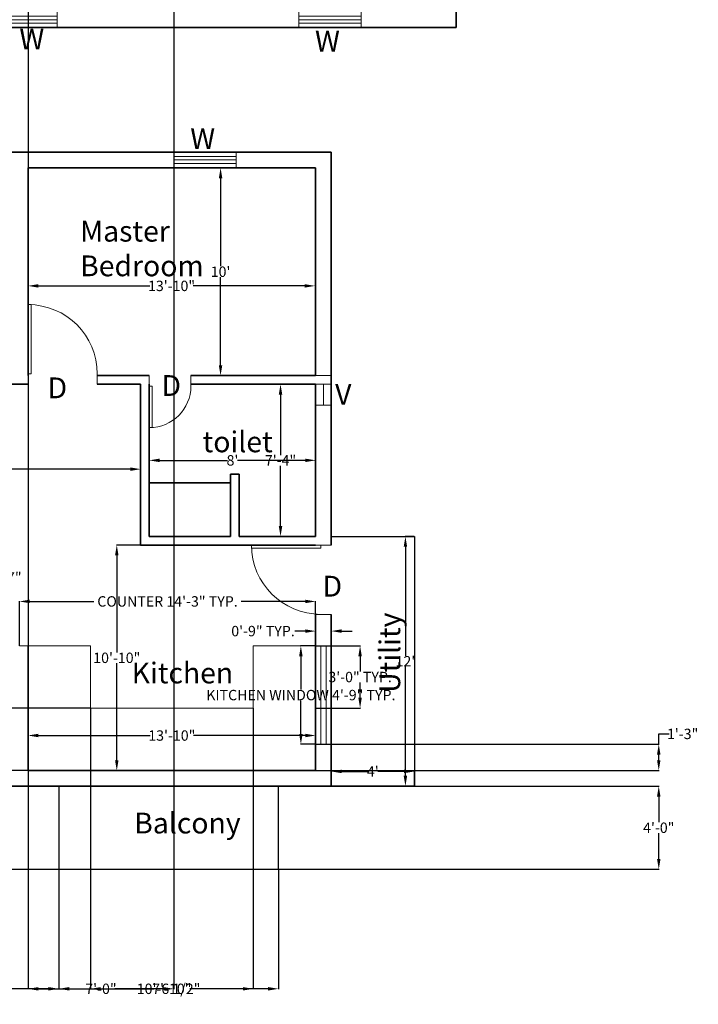
# Model space of a CAD drawing. Units: inches. Extents: x 1936 to 2761, y 1431 to 2889.
# Tile 2 of 6: x 2369 to 2761, y 1431 to 1999. Entities that reach past the tile are written whole.
import ezdxf

# ---------------------------------------------------------------- set-up
doc = ezdxf.new("R2010")
doc.units = ezdxf.units.IN
doc.header["$MEASUREMENT"] = 0
for name, color, linetype, lineweight in [('A-ANNO-DIMS', 172, 'Continuous', 13), ('A-ANNO-TEXT', 50, 'Continuous', 18), ('A-AREA-IDEN', 50, 'Continuous', 18), ('A-FLOR-EDGE', 4, 'Continuous', 25), ('A-FLOR-FIXT', 8, 'Continuous', 18), ('A-GLAZ', 3, 'Continuous', 18), ('A-WALL', 4, 'Continuous', 35), ('doors', 10, 'Continuous', 18)]:
    doc.layers.add(name, color=color, linetype=linetype, lineweight=lineweight)
doc.styles.get("Standard").update_dxf_attribs({"font": 'arial.ttf'})
doc.dimstyles.get("Standard").update_dxf_attribs({"dimtxt": 6, "dimasz": 6, "dimexe": 0.18, "dimexo": 0.0625, "dimgap": 0.09, "dimtad": 0, "dimtih": 1, "dimtoh": 1, "dimdec": 0, "dimzin": 0, "dimdsep": 46, "dimlunit": 3, "dimtxsty": 'Standard', "dimcen": 0.09, "dimadec": 0, "dimazin": 0, "dimtfac": 1, "dimtdec": 0, "dimtofl": 0, "dimtmove": 0, "dimatfit": 3, "dimfxl": 1, "dimtolj": 1, "dimtzin": 0, "dimarcsym": 0})

# ---------------------------------------------------------------- blocks, each defined once
blk = doc.blocks.new('*U2')
for p, q in [((0, 0), (0, 6)), ((40, 0), (40, 6))]:
    blk.add_line(p, q)
blk.add_lwpolyline([(0, 0), (0, -40), (1.75, -40), (1.75, 0)], close=True)
blk.add_arc((0, 0), 40, 270, 360)
blk = doc.blocks.new('*U3')
for p, q in [((0, 0), (0, -6)), ((24, 0), (24, -6))]:
    blk.add_line(p, q)
blk.add_lwpolyline([(0, 0), (0, 24), (1.75, 24), (1.75, 0)], close=True)
blk.add_arc((0, 0), 24, 0, 90)
blk = doc.blocks.new('*U5')
for p, q in [((0, 0), (0, -6)), ((40, 0), (40, -6))]:
    blk.add_line(p, q)
blk.add_lwpolyline([(0, 0), (0, 40), (1.75, 40), (1.75, 0)], close=True)
blk.add_arc((0, 0), 40, 0, 90)
blk = doc.blocks.new('*D59')
at = {"layer": 'A-ANNO-DIMS', "color": 0, "lineweight": -2, "transparency": 16777216}
for p, q in [((2249.01, 1739.61), (2249.01, 1739.73)), ((2255.01, 1739.55), (2331.56, 1739.55)), ((2433.01, 1739.55), (2356.45, 1739.55)), ((2439.01, 1739.61), (2439.01, 1739.73))]:
    blk.add_line(p, q, dxfattribs=at)
at = {"layer": 'A-ANNO-DIMS', "color": 0, "transparency": 16777216}
for points in [[(2255.01, 1740.55), (2255.01, 1738.55), (2249.01, 1739.55)], [(2433.01, 1740.55), (2433.01, 1738.55), (2439.01, 1739.55)]]:
    blk.add_solid(points, dxfattribs=at)
at = {"layer": 'Defpoints', "color": 0, "transparency": 16777216}
for p in [(2249.01, 1739.55), (2439.01, 1739.55), (2439.01, 1739.55)]:
    blk.add_point(p, dxfattribs=at)
at = {"layer": 'A-ANNO-DIMS', "color": 0, "transparency": 16777216, "insert": (2344.01, 1739.55), "char_height": 6, "attachment_point": 5}
blk.add_mtext('\\A1;15\'-10"', dxfattribs=at)
blk = doc.blocks.new('*D60')
at = {"layer": 'A-ANNO-DIMS', "color": 0, "lineweight": -2, "transparency": 16777216}
for p, q in [((2347.57, 1788.55), (2359.19, 1788.55)), ((2359.01, 1782.55), (2359.01, 1680.2)), ((2359.01, 1571.55), (2359.01, 1673.9)), ((2347.57, 1565.55), (2359.19, 1565.55))]:
    blk.add_line(p, q, dxfattribs=at)
at = {"layer": 'A-ANNO-DIMS', "color": 0, "transparency": 16777216}
for points in [[(2358.01, 1782.55), (2360.01, 1782.55), (2359.01, 1788.55)], [(2358.01, 1571.55), (2360.01, 1571.55), (2359.01, 1565.55)]]:
    blk.add_solid(points, dxfattribs=at)
at = {"layer": 'Defpoints', "color": 0, "transparency": 16777216}
for p in [(2347.51, 1788.55), (2359.01, 1788.55), (2347.51, 1565.55)]:
    blk.add_point(p, dxfattribs=at)
at = {"layer": 'A-ANNO-DIMS', "color": 0, "transparency": 16777216, "insert": (2359.01, 1677.05), "char_height": 6, "attachment_point": 5}
blk.add_mtext('\\A1;18\'-7"', dxfattribs=at)
blk = doc.blocks.new('*D61')
at = {"layer": 'A-ANNO-DIMS', "color": 0, "lineweight": -2, "transparency": 16777216}
for p, q in [((2374.01, 1585.84), (2374.01, 1585.96)), ((2380.01, 1585.78), (2444.56, 1585.78)), ((2534.01, 1585.78), (2469.45, 1585.78)), ((2540.01, 1585.84), (2540.01, 1585.96))]:
    blk.add_line(p, q, dxfattribs=at)
at = {"layer": 'A-ANNO-DIMS', "color": 0, "transparency": 16777216}
for points in [[(2380.01, 1586.78), (2380.01, 1584.78), (2374.01, 1585.78)], [(2534.01, 1586.78), (2534.01, 1584.78), (2540.01, 1585.78)]]:
    blk.add_solid(points, dxfattribs=at)
at = {"layer": 'Defpoints', "color": 0, "transparency": 16777216}
for p in [(2374.01, 1585.78), (2540.01, 1585.78), (2540.01, 1585.78)]:
    blk.add_point(p, dxfattribs=at)
at = {"layer": 'A-ANNO-DIMS', "color": 0, "transparency": 16777216, "insert": (2457.01, 1585.78), "char_height": 6, "attachment_point": 5}
blk.add_mtext('\\A1;13\'-10"', dxfattribs=at)
blk = doc.blocks.new('*D62')
at = {"layer": 'A-ANNO-DIMS', "color": 0, "lineweight": -2, "transparency": 16777216}
for p, q in [((2489.44, 1695.74), (2425.06, 1695.74)), ((2425.24, 1689.74), (2425.24, 1633.8)), ((2425.24, 1571.55), (2425.24, 1627.49)), ((2485.38, 1565.55), (2425.06, 1565.55))]:
    blk.add_line(p, q, dxfattribs=at)
at = {"layer": 'A-ANNO-DIMS', "color": 0, "transparency": 16777216}
for points in [[(2424.24, 1689.74), (2426.24, 1689.74), (2425.24, 1695.74)], [(2424.24, 1571.55), (2426.24, 1571.55), (2425.24, 1565.55)]]:
    blk.add_solid(points, dxfattribs=at)
at = {"layer": 'Defpoints', "color": 0, "transparency": 16777216}
for p in [(2425.24, 1695.74), (2489.51, 1695.74), (2485.44, 1565.55)]:
    blk.add_point(p, dxfattribs=at)
at = {"layer": 'A-ANNO-DIMS', "color": 0, "transparency": 16777216, "insert": (2425.24, 1630.64), "char_height": 6, "attachment_point": 5}
blk.add_mtext('\\A1;10\'-10"', dxfattribs=at)
blk = doc.blocks.new('*D63')
at = {"layer": 'A-ANNO-DIMS', "color": 0, "lineweight": -2, "transparency": 16777216}
for p, q in [((2444.01, 1744.58), (2444.01, 1744.46)), ((2450.01, 1744.64), (2489.15, 1744.64)), ((2534.01, 1744.64), (2494.86, 1744.64)), ((2540.01, 1744.71), (2540.01, 1744.82))]:
    blk.add_line(p, q, dxfattribs=at)
at = {"layer": 'A-ANNO-DIMS', "color": 0, "transparency": 16777216}
for points in [[(2450.01, 1745.64), (2450.01, 1743.64), (2444.01, 1744.64)], [(2534.01, 1745.64), (2534.01, 1743.64), (2540.01, 1744.64)]]:
    blk.add_solid(points, dxfattribs=at)
at = {"layer": 'Defpoints', "color": 0, "transparency": 16777216}
for p in [(2444.01, 1744.64), (2540.01, 1744.64), (2540.01, 1744.64)]:
    blk.add_point(p, dxfattribs=at)
at = {"layer": 'A-ANNO-DIMS', "color": 0, "transparency": 16777216, "insert": (2492.01, 1744.64), "char_height": 6, "attachment_point": 5}
blk.add_mtext("\\A1;8'", dxfattribs=at)
blk = doc.blocks.new('*D64')
at = {"layer": 'A-ANNO-DIMS', "color": 0, "lineweight": -2, "transparency": 16777216}
for p, q in [((2518.02, 1788.55), (2519.92, 1788.55)), ((2519.74, 1782.55), (2519.74, 1747.73)), ((2519.74, 1706.74), (2519.74, 1741.55)), ((2518.02, 1700.74), (2519.92, 1700.74))]:
    blk.add_line(p, q, dxfattribs=at)
at = {"layer": 'A-ANNO-DIMS', "color": 0, "transparency": 16777216}
for points in [[(2518.74, 1782.55), (2520.74, 1782.55), (2519.74, 1788.55)], [(2518.74, 1706.74), (2520.74, 1706.74), (2519.74, 1700.74)]]:
    blk.add_solid(points, dxfattribs=at)
at = {"layer": 'Defpoints', "color": 0, "transparency": 16777216}
for p in [(2517.96, 1788.55), (2519.74, 1788.55), (2517.96, 1700.74)]:
    blk.add_point(p, dxfattribs=at)
at = {"layer": 'A-ANNO-DIMS', "color": 0, "transparency": 16777216, "insert": (2519.74, 1744.64), "char_height": 6, "attachment_point": 5}
blk.add_mtext('\\A1;7\'-4"', dxfattribs=at)
blk = doc.blocks.new('*D73')
at = {"layer": 'A-ANNO-DIMS', "color": 0, "lineweight": -2, "transparency": 16777216}
for p, q in [((2374.01, 1858), (2374.01, 1845.18)), ((2539.69, 1858), (2539.69, 1845.18)), ((2380.01, 1845.36), (2444.41, 1845.36)), ((2533.69, 1845.36), (2469.29, 1845.36))]:
    blk.add_line(p, q, dxfattribs=at)
at = {"layer": 'A-ANNO-DIMS', "color": 0, "transparency": 16777216}
for points in [[(2380.01, 1846.36), (2380.01, 1844.36), (2374.01, 1845.36)], [(2533.69, 1846.36), (2533.69, 1844.36), (2539.69, 1845.36)]]:
    blk.add_solid(points, dxfattribs=at)
at = {"layer": 'Defpoints', "color": 0, "transparency": 16777216}
for p in [(2374.01, 1858.06), (2539.69, 1858.06), (2374.01, 1845.36)]:
    blk.add_point(p, dxfattribs=at)
at = {"layer": 'A-ANNO-DIMS', "color": 0, "transparency": 16777216, "insert": (2456.85, 1845.36), "char_height": 6, "attachment_point": 5}
blk.add_mtext('\\A1;13\'-10"', dxfattribs=at)
blk = doc.blocks.new('*D74')
at = {"layer": 'A-ANNO-DIMS', "color": 0, "lineweight": -2, "transparency": 16777216}
for p, q in [((2480.34, 1913.55), (2485.32, 1913.55)), ((2485.14, 1907.55), (2485.14, 1856.7)), ((2485.14, 1799.55), (2485.14, 1850.4)), ((2480.34, 1793.55), (2485.32, 1793.55))]:
    blk.add_line(p, q, dxfattribs=at)
at = {"layer": 'A-ANNO-DIMS', "color": 0, "transparency": 16777216}
for points in [[(2484.14, 1907.55), (2486.14, 1907.55), (2485.14, 1913.55)], [(2484.14, 1799.55), (2486.14, 1799.55), (2485.14, 1793.55)]]:
    blk.add_solid(points, dxfattribs=at)
at = {"layer": 'Defpoints', "color": 0, "transparency": 16777216}
for p in [(2480.28, 1913.55), (2480.28, 1793.55), (2485.14, 1793.55)]:
    blk.add_point(p, dxfattribs=at)
at = {"layer": 'A-ANNO-DIMS', "color": 0, "transparency": 16777216, "insert": (2485.14, 1853.55), "char_height": 6, "attachment_point": 5}
blk.add_mtext("\\A1;10'", dxfattribs=at)
blk = doc.blocks.new('*D56')
at = {"layer": 'A-ANNO-DIMS', "color": 0, "lineweight": -2, "transparency": 16777216}
for p, q in [((2549.01, 1556.61), (2549.01, 1565.24)), ((2555.01, 1565.06), (2570.03, 1565.06)), ((2591.01, 1565.06), (2575.98, 1565.06)), ((2597.01, 1556.61), (2597.01, 1565.24))]:
    blk.add_line(p, q, dxfattribs=at)
at = {"layer": 'A-ANNO-DIMS', "color": 0, "transparency": 16777216}
for points in [[(2555.01, 1566.06), (2555.01, 1564.06), (2549.01, 1565.06)], [(2591.01, 1566.06), (2591.01, 1564.06), (2597.01, 1565.06)]]:
    blk.add_solid(points, dxfattribs=at)
at = {"layer": 'Defpoints', "color": 0, "transparency": 16777216}
for p in [(2597.01, 1565.06), (2549.01, 1556.55), (2597.01, 1556.55)]:
    blk.add_point(p, dxfattribs=at)
at = {"layer": 'A-ANNO-DIMS', "color": 0, "transparency": 16777216, "insert": (2573.01, 1565.06), "char_height": 6, "attachment_point": 5}
blk.add_mtext("\\A1;4'", dxfattribs=at)
blk = doc.blocks.new('*D75')
at = {"layer": 'A-ANNO-DIMS', "color": 0, "lineweight": -2, "transparency": 16777216}
for p, q in [((2596.94, 1700.74), (2591.63, 1700.74)), ((2591.81, 1694.74), (2591.81, 1631.75)), ((2591.81, 1562.55), (2591.81, 1625.54)), ((2596.94, 1556.55), (2591.63, 1556.55))]:
    blk.add_line(p, q, dxfattribs=at)
at = {"layer": 'A-ANNO-DIMS', "color": 0, "transparency": 16777216}
for points in [[(2590.81, 1694.74), (2592.81, 1694.74), (2591.81, 1700.74)], [(2590.81, 1562.55), (2592.81, 1562.55), (2591.81, 1556.55)]]:
    blk.add_solid(points, dxfattribs=at)
at = {"layer": 'Defpoints', "color": 0, "transparency": 16777216}
for p in [(2591.81, 1700.74), (2597.01, 1700.74), (2597.01, 1556.55)]:
    blk.add_point(p, dxfattribs=at)
at = {"layer": 'A-ANNO-DIMS', "color": 0, "transparency": 16777216, "insert": (2591.81, 1628.64), "char_height": 6, "attachment_point": 5}
blk.add_mtext("\\A1;12'", dxfattribs=at)
blk = doc.blocks.new('WIN-36')
for p, q in [((0, 9), (0, 0)), ((36, 6.5), (0, 6.5)), ((36, 9), (36, 0)), ((36, 4.5), (0, 4.5)), ((36, 2.5), (0, 2.5))]:
    blk.add_line(p, q)
blk = doc.blocks.new('VENT-12')
for p, q in [((0, 0), (0, 9)), ((12, 0), (12, 9)), ((0, 4.5), (12, 4.5))]:
    blk.add_line(p, q)
blk = doc.blocks.new('WIN-KITCHEN')
for p, q in [((0, 56.83), (9, 56.83)), ((3, 56.83), (3, 0)), ((6, 56.83), (6, 0)), ((0, 0), (9, 0))]:
    blk.add_line(p, q)
blk = doc.blocks.new('COUNTER-KITCHEN-U')
for p, q in [((41, 36), (41, 0)), ((41, 36), (135, 36)), ((135, 36), (135, 0)), ((0, 0), (41, 0)), ((135, 0), (171, 0))]:
    blk.add_line(p, q)
blk = doc.blocks.new('BATH-PARTITION')
for p, q in [((0, 35.9), (46.9, 35.9)), ((0, 5), (0, 35.9)), ((46.9, 35.9), (46.9, 0)), ((51.9, 35.9), (51.9, 0)), ((46.9, 5), (0, 5)), ((51.9, 0), (46.9, 0))]:
    blk.add_line(p, q)
blk = doc.blocks.new('*D91')
at = {"layer": 'A-ANNO-DIMS', "color": 0, "lineweight": -2, "transparency": 16777216}
for p, q in [((2539.94, 1637.55), (2531.3, 1637.55)), ((2531.48, 1631.55), (2531.48, 1612.33)), ((2531.48, 1586.72), (2531.48, 1605.94)), ((2539.94, 1580.72), (2531.3, 1580.72))]:
    blk.add_line(p, q, dxfattribs=at)
at = {"layer": 'A-ANNO-DIMS', "color": 0, "transparency": 16777216}
for points in [[(2530.48, 1631.55), (2532.48, 1631.55), (2531.48, 1637.55)], [(2530.48, 1586.72), (2532.48, 1586.72), (2531.48, 1580.72)]]:
    blk.add_solid(points, dxfattribs=at)
at = {"layer": 'Defpoints', "color": 0, "transparency": 16777216}
for p in [(2540.01, 1637.55), (2531.48, 1580.72), (2540.01, 1580.72)]:
    blk.add_point(p, dxfattribs=at)
at = {"layer": 'A-ANNO-DIMS', "color": 0, "transparency": 16777216, "insert": (2531.48, 1609.13), "char_height": 6, "attachment_point": 5}
blk.add_mtext('\\A1;KITCHEN WINDOW 4\'-9" TYP.', dxfattribs=at)
blk = doc.blocks.new('*D92')
at = {"layer": 'A-ANNO-DIMS', "color": 0, "lineweight": -2, "transparency": 16777216}
for p, q in [((2534.01, 1646.07), (2528.01, 1646.07)), ((2540.01, 1637.61), (2540.01, 1646.25)), ((2549.01, 1637.61), (2549.01, 1646.25)), ((2555.01, 1646.07), (2561.01, 1646.07))]:
    blk.add_line(p, q, dxfattribs=at)
at = {"layer": 'A-ANNO-DIMS', "color": 0, "transparency": 16777216}
for points in [[(2534.01, 1647.07), (2534.01, 1645.07), (2540.01, 1646.07)], [(2555.01, 1647.07), (2555.01, 1645.07), (2549.01, 1646.07)]]:
    blk.add_solid(points, dxfattribs=at)
at = {"layer": 'Defpoints', "color": 0, "transparency": 16777216}
for p in [(2540.01, 1646.07), (2540.01, 1637.55), (2549.01, 1637.55)]:
    blk.add_point(p, dxfattribs=at)
at = {"layer": 'A-ANNO-DIMS', "color": 0, "transparency": 16777216, "insert": (2509.63, 1646.07), "char_height": 6, "attachment_point": 5}
blk.add_mtext('\\A1;0\'-9" TYP.', dxfattribs=at)
blk = doc.blocks.new('*D93')
at = {"layer": 'A-ANNO-DIMS', "color": 0, "lineweight": -2, "transparency": 16777216}
for p, q in [((2369.01, 1637.61), (2369.01, 1663.38)), ((2375.01, 1663.2), (2411.95, 1663.2)), ((2534.01, 1663.2), (2497.06, 1663.2)), ((2540.01, 1637.61), (2540.01, 1663.38))]:
    blk.add_line(p, q, dxfattribs=at)
at = {"layer": 'A-ANNO-DIMS', "color": 0, "transparency": 16777216}
for points in [[(2375.01, 1664.2), (2375.01, 1662.2), (2369.01, 1663.2)], [(2534.01, 1664.2), (2534.01, 1662.2), (2540.01, 1663.2)]]:
    blk.add_solid(points, dxfattribs=at)
at = {"layer": 'Defpoints', "color": 0, "transparency": 16777216}
for p in [(2540.01, 1663.2), (2369.01, 1637.55), (2540.01, 1637.55)]:
    blk.add_point(p, dxfattribs=at)
at = {"layer": 'A-ANNO-DIMS', "color": 0, "transparency": 16777216, "insert": (2454.51, 1663.2), "char_height": 6, "attachment_point": 5}
blk.add_mtext('\\A1;COUNTER 14\'-3" TYP.', dxfattribs=at)
blk = doc.blocks.new('*D94')
at = {"layer": 'A-ANNO-DIMS', "color": 0, "lineweight": -2, "transparency": 16777216}
for p, q in [((2540.07, 1637.55), (2565.84, 1637.55)), ((2565.66, 1631.55), (2565.66, 1622.7)), ((2565.66, 1607.55), (2565.66, 1616.39)), ((2540.07, 1601.55), (2565.84, 1601.55))]:
    blk.add_line(p, q, dxfattribs=at)
at = {"layer": 'A-ANNO-DIMS', "color": 0, "transparency": 16777216}
for points in [[(2564.66, 1631.55), (2566.66, 1631.55), (2565.66, 1637.55)], [(2564.66, 1607.55), (2566.66, 1607.55), (2565.66, 1601.55)]]:
    blk.add_solid(points, dxfattribs=at)
at = {"layer": 'Defpoints', "color": 0, "transparency": 16777216}
for p in [(2540.01, 1637.55), (2540.01, 1601.55), (2565.66, 1601.55)]:
    blk.add_point(p, dxfattribs=at)
at = {"layer": 'A-ANNO-DIMS', "color": 0, "transparency": 16777216, "insert": (2565.66, 1619.55), "char_height": 6, "attachment_point": 5}
blk.add_mtext('\\A1;3\'-0" TYP.', dxfattribs=at)
blk = doc.blocks.new('*D101')
at = {"layer": 'A-ANNO-DIMS', "color": 0, "lineweight": -2, "transparency": 16777216}
for p, q in [((2391.78, 1508.49), (2391.78, 1439.37)), ((2518.49, 1508.49), (2518.49, 1439.37)), ((2397.78, 1439.55), (2438.03, 1439.55)), ((2512.49, 1439.55), (2472.24, 1439.55))]:
    blk.add_line(p, q, dxfattribs=at)
at = {"layer": 'A-ANNO-DIMS', "color": 0, "transparency": 16777216}
for points in [[(2397.78, 1440.55), (2397.78, 1438.55), (2391.78, 1439.55)], [(2512.49, 1440.55), (2512.49, 1438.55), (2518.49, 1439.55)]]:
    blk.add_solid(points, dxfattribs=at)
at = {"layer": 'Defpoints', "color": 0, "transparency": 16777216}
for p in [(2391.78, 1508.55), (2518.49, 1508.55), (2518.49, 1439.55)]:
    blk.add_point(p, dxfattribs=at)
at = {"layer": 'A-ANNO-DIMS', "color": 0, "transparency": 16777216, "insert": (2455.14, 1439.55), "char_height": 6, "attachment_point": 5}
blk.add_mtext('\\A1;10\'-6 1/2"', dxfattribs=at)
blk = doc.blocks.new('*D102')
at = {"layer": 'A-ANNO-DIMS', "color": 0, "lineweight": -2, "transparency": 16777216}
for p, q in [((2150.85, 1556.55), (2738.19, 1556.55)), ((2738.01, 1550.55), (2738.01, 1535.7)), ((2738.01, 1514.55), (2738.01, 1529.4)), ((2150.85, 1508.55), (2738.19, 1508.55))]:
    blk.add_line(p, q, dxfattribs=at)
at = {"layer": 'A-ANNO-DIMS', "color": 0, "transparency": 16777216}
for points in [[(2737.01, 1550.55), (2739.01, 1550.55), (2738.01, 1556.55)], [(2737.01, 1514.55), (2739.01, 1514.55), (2738.01, 1508.55)]]:
    blk.add_solid(points, dxfattribs=at)
at = {"layer": 'Defpoints', "color": 0, "transparency": 16777216}
for p in [(2150.78, 1556.55), (2738.01, 1556.55), (2150.78, 1508.55)]:
    blk.add_point(p, dxfattribs=at)
at = {"layer": 'A-ANNO-DIMS', "color": 0, "transparency": 16777216, "insert": (2738.01, 1532.55), "char_height": 6, "attachment_point": 5}
blk.add_mtext('\\A1;4\'-0"', dxfattribs=at)
blk = doc.blocks.new('*D103')
at = {"layer": 'A-ANNO-DIMS', "color": 0, "lineweight": -2, "transparency": 16777216}
for p, q in [((2150.78, 1508.49), (2150.78, 1439.37)), ((2391.78, 1508.49), (2391.78, 1439.37)), ((2156.78, 1439.55), (2260.84, 1439.55)), ((2385.78, 1439.55), (2281.73, 1439.55))]:
    blk.add_line(p, q, dxfattribs=at)
at = {"layer": 'A-ANNO-DIMS', "color": 0, "transparency": 16777216}
for points in [[(2156.78, 1440.55), (2156.78, 1438.55), (2150.78, 1439.55)], [(2385.78, 1440.55), (2385.78, 1438.55), (2391.78, 1439.55)]]:
    blk.add_solid(points, dxfattribs=at)
at = {"layer": 'Defpoints', "color": 0, "transparency": 16777216}
for p in [(2150.78, 1508.55), (2391.78, 1508.55), (2391.78, 1439.55)]:
    blk.add_point(p, dxfattribs=at)
at = {"layer": 'A-ANNO-DIMS', "color": 0, "transparency": 16777216, "insert": (2271.28, 1439.55), "char_height": 6, "attachment_point": 5}
blk.add_mtext('\\A1;20\'-1"', dxfattribs=at)
blk = doc.blocks.new('*D112')
at = {"layer": 'A-ANNO-DIMS', "color": 0, "lineweight": -2, "transparency": 16777216}
for p, q in [((2374.01, 2459.49), (2374.01, 1439.37)), ((2458.21, 2459.49), (2458.21, 1439.37)), ((2380.01, 1439.55), (2408.07, 1439.55)), ((2452.21, 1439.55), (2424.15, 1439.55))]:
    blk.add_line(p, q, dxfattribs=at)
at = {"layer": 'A-ANNO-DIMS', "color": 0, "transparency": 16777216}
for points in [[(2380.01, 1440.55), (2380.01, 1438.55), (2374.01, 1439.55)], [(2452.21, 1440.55), (2452.21, 1438.55), (2458.21, 1439.55)]]:
    blk.add_solid(points, dxfattribs=at)
at = {"layer": 'Defpoints', "color": 0, "transparency": 16777216}
for p in [(2374.01, 2459.55), (2458.21, 2459.55), (2458.21, 1439.55)]:
    blk.add_point(p, dxfattribs=at)
at = {"layer": 'A-ANNO-DIMS', "color": 0, "transparency": 16777216, "insert": (2416.11, 1439.55), "char_height": 6, "attachment_point": 5}
blk.add_mtext('\\A1;7\'-0"', dxfattribs=at)
blk = doc.blocks.new('*D115')
at = {"layer": 'A-ANNO-DIMS', "color": 0, "lineweight": -2, "transparency": 16777216}
for p, q in [((2738.01, 1580.72), (2738.01, 1586.72)), ((2738.01, 1586.72), (2744.01, 1586.72)), ((2540.07, 1580.72), (2738.19, 1580.72)), ((2738.01, 1571.55), (2738.01, 1574.72)), ((2540.07, 1565.55), (2738.19, 1565.55))]:
    blk.add_line(p, q, dxfattribs=at)
at = {"layer": 'A-ANNO-DIMS', "color": 0, "transparency": 16777216}
for points in [[(2737.01, 1574.72), (2739.01, 1574.72), (2738.01, 1580.72)], [(2737.01, 1571.55), (2739.01, 1571.55), (2738.01, 1565.55)]]:
    blk.add_solid(points, dxfattribs=at)
at = {"layer": 'Defpoints', "color": 0, "transparency": 16777216}
for p in [(2540.01, 1580.72), (2738.01, 1580.72), (2540.01, 1565.55)]:
    blk.add_point(p, dxfattribs=at)
at = {"layer": 'A-ANNO-DIMS', "color": 0, "transparency": 16777216, "insert": (2751.79, 1586.72), "char_height": 6, "attachment_point": 5}
blk.add_mtext('\\A1;1\'-3"', dxfattribs=at)
blk = doc.blocks.new('*D116')
at = {"layer": 'A-ANNO-DIMS', "color": 0, "lineweight": -2, "transparency": 16777216}
for p, q in [((2410.01, 1601.49), (2410.01, 1439.37)), ((2504.01, 1601.49), (2504.01, 1439.37)), ((2416.01, 1439.55), (2446.64, 1439.55)), ((2498.01, 1439.55), (2467.38, 1439.55))]:
    blk.add_line(p, q, dxfattribs=at)
at = {"layer": 'A-ANNO-DIMS', "color": 0, "transparency": 16777216}
for points in [[(2416.01, 1440.55), (2416.01, 1438.55), (2410.01, 1439.55)], [(2498.01, 1440.55), (2498.01, 1438.55), (2504.01, 1439.55)]]:
    blk.add_solid(points, dxfattribs=at)
at = {"layer": 'Defpoints', "color": 0, "transparency": 16777216}
for p in [(2410.01, 1601.55), (2504.01, 1601.55), (2504.01, 1439.55)]:
    blk.add_point(p, dxfattribs=at)
at = {"layer": 'A-ANNO-DIMS', "color": 0, "transparency": 16777216, "insert": (2457.01, 1439.55), "char_height": 6, "attachment_point": 5}
blk.add_mtext('\\A1;7\'-10"', dxfattribs=at)
blk = doc.blocks.new('*D117')
at = {"layer": 'A-ANNO-DIMS', "color": 0, "lineweight": -2, "transparency": 16777216}
for p, q in [((2409.94, 1601.55), (1951.83, 1601.55)), ((1952.01, 1595.55), (1952.01, 1586.7)), ((1952.01, 1571.55), (1952.01, 1580.39)), ((2373.94, 1565.55), (1951.83, 1565.55))]:
    blk.add_line(p, q, dxfattribs=at)
at = {"layer": 'A-ANNO-DIMS', "color": 0, "transparency": 16777216}
for points in [[(1951.01, 1595.55), (1953.01, 1595.55), (1952.01, 1601.55)], [(1951.01, 1571.55), (1953.01, 1571.55), (1952.01, 1565.55)]]:
    blk.add_solid(points, dxfattribs=at)
at = {"layer": 'Defpoints', "color": 0, "transparency": 16777216}
for p in [(1952.01, 1601.55), (2410.01, 1601.55), (2374.01, 1565.55)]:
    blk.add_point(p, dxfattribs=at)
at = {"layer": 'A-ANNO-DIMS', "color": 0, "transparency": 16777216, "insert": (1952.01, 1583.55), "char_height": 6, "attachment_point": 5}
blk.add_mtext('\\A1;3\'-0"', dxfattribs=at)

msp = doc.modelspace()

# ---------------------------------------------------------------- linework, layer by layer
at = {"layer": 'A-FLOR-EDGE'}
for p, q in [((2549.01, 1700.74), (2597.01, 1700.74)), ((2597.01, 1700.74), (2597.01, 1556.55)), ((2391.78, 1556.55), (2391.78, 1508.55)), ((2518.49, 1508.55), (2518.49, 1556.55)), ((2391.78, 1508.55), (2518.49, 1508.55))]:
    msp.add_line(p, q, dxfattribs=at)
at = {"layer": 'A-WALL'}
for p, q in [((2621.01, 2083.55), (2621.01, 1994.55)), ((2621.01, 1994.55), (2141.01, 1994.55)), ((2549.01, 1922.55), (2069.01, 1922.55)), ((2549.01, 1793.55), (2549.01, 1922.55)), ((2374.01, 1793.55), (2374.01, 1913.55)), ((2540.01, 1913.55), (2374.01, 1913.55)), ((2540.01, 1793.55), (2540.01, 1913.55)), ((2444.01, 1793.55), (2414.01, 1793.55)), ((2540.01, 1793.55), (2468.01, 1793.55)), ((2549.01, 1695.74), (2549.01, 1793.55)), ((2374.01, 1788.55), (2289.01, 1788.55)), ((2439.01, 1788.55), (2414.01, 1788.55)), ((2439.01, 1695.74), (2439.01, 1788.55)), ((2444.01, 1700.74), (2444.01, 1788.55)), ((2540.01, 1788.55), (2468.01, 1788.55)), ((2540.01, 1700.74), (2540.01, 1788.55)), ((2444.01, 1700.74), (2490.9, 1700.74)), ((2495.9, 1700.74), (2540.01, 1700.74)), ((2439.01, 1695.74), (2540.01, 1695.74)), ((2540.01, 1565.55), (2540.01, 1655.74)), ((2549.01, 1556.55), (2549.01, 1655.74)), ((2374.01, 1565.55), (2374.01, 1637.55)), ((2374.01, 1565.55), (2540.01, 1565.55)), ((2069.01, 1556.55), (2597.01, 1556.55))]:
    msp.add_line(p, q, dxfattribs=at)
at = {"layer": 'doors'}
for p, q in [((2374.01, 1788.55), (2374.01, 1793.55)), ((2414.01, 1788.55), (2414.01, 1793.55)), ((2444.01, 1788.55), (2444.01, 1793.55)), ((2468.01, 1788.55), (2468.01, 1793.55)), ((2540.01, 1793.55), (2549.01, 1793.55)), ((2540.01, 1695.74), (2549.01, 1695.74)), ((2540.01, 1655.74), (2549.01, 1655.74))]:
    msp.add_line(p, q, dxfattribs=at)

# ---------------------------------------------------------------- block references
at = {"layer": 'A-FLOR-FIXT', "extrusion": (0, 0, -1), "zscale": -1, "rotation": 180}
msp.add_blockref('COUNTER-KITCHEN-U', (-2369.01, 1637.55), dxfattribs=at)
at = {"layer": 'A-GLAZ'}
for p in [(2354.92, 1994.55), (2530.21, 1994.55), (2458.21, 1913.55)]:
    msp.add_blockref('WIN-36', p, dxfattribs=at)
for name, p, rotation in [('VENT-12', (2549.01, 1776.55), 89.99999999999618), ('WIN-KITCHEN', (2549.01, 1637.55), 180)]:
    msp.add_blockref(name, p, dxfattribs=dict(at, rotation=rotation))
at = {"layer": 'A-WALL', "extrusion": (0, 0, -1), "zscale": -1, "rotation": 180}
msp.add_blockref('BATH-PARTITION', (-2444.01, 1736.64), dxfattribs=at)
at = {"layer": 'doors', "xscale": -1}
for name, p, rotation in [('*U2', (2374.01, 1794.55), 180), ('*U3', (2444.01, 1787.55), 180), ('*U5', (2543.01, 1695.74), 90)]:
    msp.add_blockref(name, p, dxfattribs=dict(at, rotation=rotation))

# ---------------------------------------------------------------- texts
at = {"layer": 'A-ANNO-TEXT', "char_height": 12}
for s, width, heights, insert, attachment_point in [('W', 7.8209, [0.2], (2369.01, 1993.85), 1), ('W', 7.8209, [0.2], (2539.63, 1992.68), 1), ('W', 7.8209, [0.2], (2467.63, 1924.42), 7), ('D', 28.2371, [0.2], (2385.33, 1780.49), 7), ('D', 28.2371, [0.2], (2451.04, 1781.85), 7), ('V', 13.1151, [0], (2551.24, 1776.73), 7), ('D', 28.2371, [0.2], (2544.03, 1665.99), 7)]:
    msp.add_mtext_dynamic_manual_height_columns(s, width=width, gutter_width=1, heights=heights, dxfattribs=dict(at, insert=insert, attachment_point=attachment_point))
at = {"layer": 'A-AREA-IDEN', "char_height": 12}
for s, insert, attachment_point in [('Master Bedroom', (2404.08, 1850.93), 7), ('toilet', (2474.76, 1749.33), 7), ('Kitchen', (2433.82, 1615.9), 7), ('Balcony', (2435.29, 1541.24), 1)]:
    msp.add_mtext_dynamic_manual_height_columns(s, width=55.7076, gutter_width=1, heights=[0], dxfattribs=dict(at, insert=insert, attachment_point=attachment_point))
at = {"layer": 'A-AREA-IDEN', "insert": (2576.79, 1656.75), "char_height": 12, "attachment_point": 3, "rotation": 90}
msp.add_mtext_dynamic_manual_height_columns('Utility', width=55.7076, gutter_width=1, heights=[0], dxfattribs=at)

# ---------------------------------------------------------------- dimensions: what is measured, and where the dimension line sits
at = {"layer": 'A-ANNO-DIMS'}
for base, p1, p2, override, picture, middle in [((2458.21, 1439.55), (2374.01, 2459.55), (2458.21, 2459.55), {"dimdec": 1, "dimlfac": 1, "dimrnd": 0, "dimzin": 1, "dimdsep": 46, "dimlunit": 4, "dimfrac": 2}, '*D112', (2416.11, 1439.55)), ((2374.01, 1845.36), (2539.69, 1858.06), (2374.01, 1858.06), {"dimclrd": 0, "dimclre": 0, "dimclrt": 0}, '*D73', (2456.85, 1845.36)), ((2540.01, 1744.64), (2444.01, 1744.64), (2540.01, 1744.64), {"dimclrd": 0, "dimclre": 0, "dimclrt": 0}, '*D63', (2492.01, 1744.64)), ((2439.01, 1739.55), (2249.01, 1739.55), (2439.01, 1739.55), {"dimclrd": 0, "dimclre": 0, "dimclrt": 0}, '*D59', (2344.01, 1739.55)), ((2504.01, 1439.55), (2410.01, 1601.55), (2504.01, 1601.55), {"dimdec": 1, "dimlfac": 1, "dimrnd": 0, "dimzin": 1, "dimdsep": 46, "dimlunit": 4, "dimfrac": 2}, '*D116', (2457.01, 1439.55)), ((2540.01, 1585.78), (2374.01, 1585.78), (2540.01, 1585.78), {"dimclrd": 0, "dimclre": 0, "dimclrt": 0}, '*D61', (2457.01, 1585.78)), ((2597.01, 1565.06), (2549.01, 1556.55), (2597.01, 1556.55), {"dimclrd": 0, "dimclre": 0, "dimclrt": 0}, '*D56', (2573.01, 1565.06)), ((2391.78, 1439.55), (2150.78, 1508.55), (2391.78, 1508.55), {"dimdec": 1, "dimlfac": 1, "dimrnd": 0, "dimzin": 1, "dimdsep": 46, "dimlunit": 4, "dimfrac": 2}, '*D103', (2271.28, 1439.55)), ((2518.49, 1439.55), (2391.78, 1508.55), (2518.49, 1508.55), {"dimdec": 1, "dimlfac": 1, "dimrnd": 0, "dimzin": 1, "dimdsep": 46, "dimlunit": 4, "dimfrac": 2}, '*D101', (2455.14, 1439.55))]:
    dim = msp.add_linear_dim(base=base, p1=p1, p2=p2, dimstyle='Standard', override=override, dxfattribs=at)
    dim.commit()
    dim.dimension.update_dxf_attribs({"geometry": picture, "text_midpoint": middle})
for base, p1, p2, angle, override, picture, middle in [((2485.14, 1793.55), (2480.28, 1913.55), (2480.28, 1793.55), 270, {"dimclrd": 0, "dimclre": 0, "dimclrt": 0}, '*D74', (2485.14, 1853.55)), ((2359.01, 1788.55), (2347.51, 1565.55), (2347.51, 1788.55), 270, {"dimclrd": 0, "dimclre": 0, "dimclrt": 0}, '*D60', (2359.01, 1677.05)), ((2519.74, 1788.55), (2517.96, 1700.74), (2517.96, 1788.55), 270, {"dimclrd": 0, "dimclre": 0, "dimclrt": 0}, '*D64', (2519.74, 1744.64)), ((2591.81, 1700.74), (2597.01, 1556.55), (2597.01, 1700.74), 270, {"dimclrd": 0, "dimclre": 0, "dimclrt": 0}, '*D75', (2591.81, 1628.64)), ((2425.24, 1695.74), (2485.44, 1565.55), (2489.51, 1695.74), 270, {"dimclrd": 0, "dimclre": 0, "dimclrt": 0}, '*D62', (2425.24, 1630.64)), ((1952.01, 1601.55), (2374.01, 1565.55), (2410.01, 1601.55), 90, {"dimdec": 1, "dimlfac": 1, "dimrnd": 0, "dimzin": 1, "dimdsep": 46, "dimlunit": 4, "dimfrac": 2}, '*D117', (1952.01, 1583.55)), ((2738.01, 1580.72), (2540.01, 1565.55), (2540.01, 1580.72), 90, {"dimdec": 1, "dimlfac": 1, "dimrnd": 0, "dimzin": 1, "dimdsep": 46, "dimlunit": 4, "dimfrac": 2}, '*D115', (2751.79, 1586.72)), ((2738.01, 1556.55), (2150.78, 1508.55), (2150.78, 1556.55), 90, {"dimdec": 1, "dimlfac": 1, "dimrnd": 0, "dimzin": 1, "dimdsep": 46, "dimlunit": 4, "dimfrac": 2}, '*D102', (2738.01, 1532.55))]:
    dim = msp.add_linear_dim(base=base, p1=p1, p2=p2, angle=angle, dimstyle='Standard', override=override, dxfattribs=at)
    dim.commit()
    dim.dimension.update_dxf_attribs({"geometry": picture, "text_midpoint": middle})
dim = msp.add_linear_dim(base=(2540.01, 1663.2), p1=(2369.01, 1637.55), p2=(2540.01, 1637.55), text='COUNTER <> TYP.', dimstyle='Standard', override={"dimdec": 1, "dimlfac": 1, "dimrnd": 0, "dimzin": 1, "dimdsep": 46, "dimlunit": 4, "dimfrac": 2}, dxfattribs=at)
dim.commit()
dim.dimension.update_dxf_attribs({"geometry": '*D93', "text_midpoint": (2454.51, 1663.2)})
for base, p1, p2, angle, text, picture, middle in [((2540.01, 1646.07), (2549.01, 1637.55), (2540.01, 1637.55), 180, '<> TYP.', '*D92', (2509.63, 1646.07)), ((2531.48, 1580.72), (2540.01, 1637.55), (2540.01, 1580.72), 270, 'KITCHEN WINDOW <> TYP.', '*D91', (2531.48, 1609.13)), ((2565.66, 1601.55), (2540.01, 1637.55), (2540.01, 1601.55), 270, '<> TYP.', '*D94', (2565.66, 1619.55))]:
    dim = msp.add_linear_dim(base=base, p1=p1, p2=p2, angle=angle, text=text, dimstyle='Standard', override={"dimdec": 1, "dimlfac": 1, "dimrnd": 0, "dimzin": 1, "dimdsep": 46, "dimlunit": 4, "dimfrac": 2}, dxfattribs=at)
    dim.commit()
    dim.dimension.update_dxf_attribs({"geometry": picture, "text_midpoint": middle})

doc.saveas('drawing.dxf')
